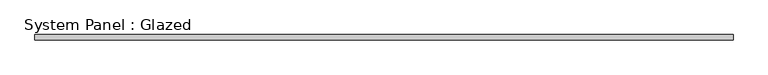
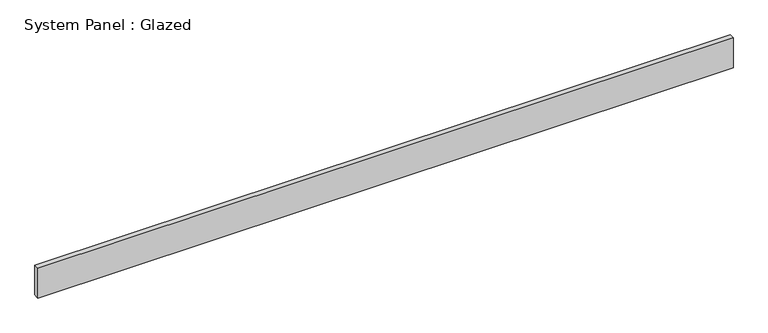
"""IFC4 building model written with IfcOpenShell, lengths in millimetres: plate geometry, System Panel : Glazed."""

from ifc_helpers import new_model, si_unit, origin, origin_with_axes, place, context, project, spatial, polyline, outline, extrude, source, transform, mapped, element, save


def system_panel_glazed_61df8711(model_context):
    return source(origin(), model_context, "Body", "SweptSolid", [
        extrude(outline(polyline([(1676.4, 19.05), (-1676.4, 19.05), (-1676.4, 44.45), (1676.4, 44.45), (1676.4, 19.05)])), origin_with_axes(), (0.0, 0.0, 1.0), 152.4),
    ])


if __name__ == "__main__":
    model = new_model("IFC4")
    model_context = context("Model", 3, world=origin())
    ifc_project = project(units=[si_unit("LENGTHUNIT", "METRE", prefix="MILLI")], contexts=[model_context])
    site = spatial("IfcSite", under=ifc_project)
    building = spatial("IfcBuilding", under=site)
    placement = place(None, origin())
    system_panel_glazed_shape = system_panel_glazed_61df8711(model_context)
    element("IfcPlate", 1, ObjectType="System Panel : Glazed", at=placement, inside=building, context=model_context, shape_type="MappedRepresentation", body=[
        mapped(system_panel_glazed_shape, transform((0.0, 0.0, 0.0), x_axis=(1.0, 0.0, 0.0), y_axis=(0.0, 1.0, 0.0), z_axis=(0.0, 0.0, 1.0))),
    ])
    save(model, "model.ifc")

# Revit data of these elements
# Type "System Panel : Glazed"
#   Construction Type Id = "GSP4R"
#   Analytic Construction = "1/8 in Pilkington single glazing"
#   Visual Light Transmittance = 0.9
#   Solar Heat Gain Coefficient = 0.86
#   Heat Transfer Coefficient (U) = 1.18115 BTU/(h·ft²·°F)
#   Define Thermal Properties by = 1
# Element 1 (IfcPlate, "System Panel : Glazed")
#   Materials on its faces: "Glass"
# Materials
#   "Glass": class "Glass", colour RGB 0 128 192, transparency 0.75, Description = "Soda Lime Glass", Cost = 0
